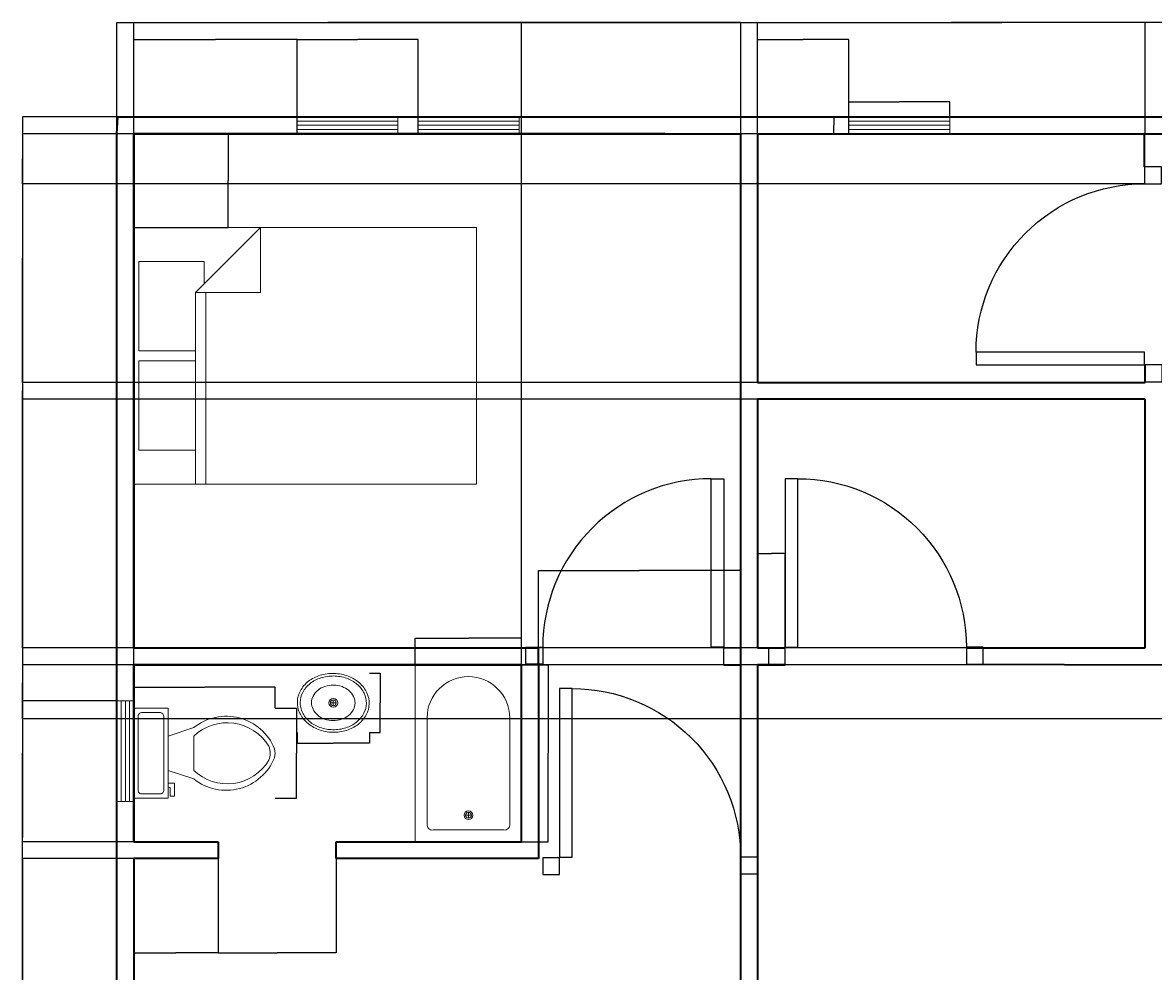
# Model space of a CAD drawing. Units: millimetres. Extents: x 1312 to 12932, y -881 to 10062.
# Tile 2 of 4: x 1312 to 8020, y 4434 to 10062. Entities that reach past the tile are written whole.
import ezdxf

# ---------------------------------------------------------------- set-up
doc = ezdxf.new("R2010")
doc.units = ezdxf.units.MM
for name, color, linetype, lineweight in [('A-ANNO-DIMS', 2, 'Continuous', 18), ('A-DOOR', 3, 'Continuous', 25), ('A-FLOR-FIXT', 9, 'Continuous', 18), ('A-FURN', 8, 'Continuous', 18), ('A-GLAZ', 4, 'Continuous', 18), ('A-WALL', 7, 'Continuous', 35)]:
    doc.layers.add(name, color=color, linetype=linetype, lineweight=lineweight)
doc.styles.get("Standard").update_dxf_attribs({"font": 'arial.ttf'})
doc.dimstyles.get("Standard").update_dxf_attribs({"dimtxt": 0.18, "dimasz": 0.18, "dimexe": 0.18, "dimexo": 0.0625, "dimgap": 0.09, "dimtad": 0, "dimtih": 1, "dimtoh": 1, "dimdec": 4, "dimzin": 0, "dimdsep": 46, "dimtxsty": 'Standard', "dimcen": 0.09, "dimadec": 0, "dimazin": 0, "dimtfac": 1, "dimtdec": 4, "dimtofl": 0, "dimtmove": 0, "dimatfit": 3, "dimfxl": 1, "dimtolj": 1, "dimtzin": 0, "dimarcsym": 0})

# ---------------------------------------------------------------- blocks, each defined once
blk = doc.blocks.new('Toilet - top')
for p, q in [((9.5, -6), (9.5, -2)), ((-10, -8.5), (-8, -8.5)), ((-10, -9.5), (-10, -8.5)), ((-7, -9.5), (-10, -9.5)), ((-8, -8.5), (-8, -8)), ((-7, -8), (-7, -9.5)), ((-4, -8), (-6, -14)), ((4, -8), (6, -14)), ((4, -14), (-4, -14))]:
    blk.add_line(p, q)
blk.add_lwpolyline([(10.5, -8), (10.5, 0), (-10.5, 0), (-10.5, -8)], close=True)
for points in [[(-9.5, -2), (-9.5, -6)], [(8.5, -1), (-8.5, -1)], [(-8.5, -7), (8.5, -7)]]:
    blk.add_lwpolyline(points)
for centre, radius, start, end in [((-8.62, -1.88), 0.884, 81.8699, 188.1301), ((8.62, -1.88), 0.884, 351.8699, 98.1301), ((-8.62, -6.12), 0.884, 171.8699, 278.1301), ((8.62, -6.12), 0.884, 261.8699, 8.1301), ((3.52, -21.58), 12.17, 141.4691, 247.9714), ((4.2, -21.82), 11.33, 136.3677, 238.9468), ((-3.52, -21.58), 12.17, 292.0284, 38.5307), ((-4.2, -21.82), 11.33, 301.053, 43.6321), ((0, -27.88), 4, 245.7318, 294.2682), ((0, -29), 4, 254.8605, 285.1395)]:
    blk.add_arc(centre, radius, start, end)
blk = doc.blocks.new('Bath Tub - 26 x 60 in.')
for p, q in [((8, -18), (10, -18)), ((9, -17), (9, -19))]:
    blk.add_line(p, q)
blk.add_lwpolyline([(0, -36), (0, 0), (60, 0), (60, -36)], close=True)
for points in [[(4, -30), (4, -6)], [(6, -4), (42, -4)], [(42, -32), (6, -32)]]:
    blk.add_lwpolyline(points)
for radius in [1.5, 1]:
    blk.add_circle((9, -18), radius)
for centre, radius, start, end in [((5.75, -5.75), 1.77, 81.8699, 188.1301), ((42, -18), 14, 270, 90), ((5.75, -30.25), 1.77, 171.8699, 278.1301)]:
    blk.add_arc(centre, radius, start, end)
blk = doc.blocks.new('Bed - Queen')
for p, q in [((0, -80.00003), (0, 0)), ((0, 0), (59.99999, 0)), ((59.99999, 0), (59.99999, -80.00003)), ((7.99999, -1.2), (28.79998, -1.2)), ((7.99999, -14.4), (7.99999, -1.2)), ((28.79998, -1.2), (28.79998, -14.4)), ((31.19999, -1.2), (51.99999, -1.2)), ((31.19999, -14.4), (31.19999, -1.2)), ((51.99999, -1.2), (51.99999, -16.4)), ((0, -14.4), (44.8, -14.4)), ((59.99999, -29.6), (44.8, -14.4)), ((44.8, -14.4), (44.8, -29.6)), ((44.8, -16.8), (0, -16.8)), ((51.99999, -16.4), (46.79936, -16.4)), ((44.8, -29.6), (59.99999, -29.6)), ((59.99999, -80.00003), (0, -80.00003))]:
    blk.add_line(p, q)
blk = doc.blocks.new('Sink - Oval top')
for p, q in [((-1, 0), (1, 0)), ((0, 1), (0, -1))]:
    blk.add_line(p, q)
for points in [[(-12.23, 0.39, 0.117634), (-11.46, -3.36, 0.104469), (-8.88, -6.8, 0.090016), (-5.08, -9.07, 0.08192), (-0.32, -10.02, 0.08192), (4.49, -9.38, 0.090016), (8.42, -7.36, 0.104469), (11.22, -4.09, 0.117634), (12.23, -0.39, 0.117634), (11.46, 3.36, 0.104469), (8.88, 6.8, 0.090016), (5.08, 9.07, 0.08192), (0.32, 10.02, 0.08192), (-4.49, 9.38, 0.090016), (-8.42, 7.36, 0.104469), (-11.22, 4.09, 0.117634)], [(-11.29, 0.16, 0.118622), (-10.52, -3.25, 0.104678), (-8.07, -6.36, 0.089562), (-4.54, -8.37, 0.081185), (-0.13, -9.15, 0.081185), (4.3, -8.49, 0.089562), (7.89, -6.58, 0.104678), (10.42, -3.55, 0.118622), (11.29, -0.16, 0.118622), (10.52, 3.25, 0.104678), (8.07, 6.36, 0.089562), (4.54, 8.37, 0.081185), (0.13, 9.15, 0.081185), (-4.3, 8.49, 0.089562), (-7.89, 6.58, 0.104678), (-10.42, 3.55, 0.118622)], [(-7.42, 0.08, 0.118283), (-6.91, -2.17, 0.104607), (-5.29, -4.21, 0.089718), (-2.97, -5.53, 0.081436), (-0.07, -6.04, 0.081436), (2.84, -5.59, 0.089718), (5.2, -4.33, 0.104607), (6.86, -2.32, 0.118283), (7.42, -0.08, 0.118283), (6.91, 2.17, 0.104607), (5.29, 4.21, 0.089718), (2.97, 5.53, 0.081436), (0.07, 6.04, 0.081436), (-2.84, 5.59, 0.089718), (-5.2, 4.33, 0.104607), (-6.86, 2.32, 0.118283)]]:
    blk.add_lwpolyline(points, format="xyb", close=True)
for radius in [1.5, 1]:
    blk.add_circle((0, 0), radius)
blk = doc.blocks.new('Window - Wood Frame 36 in. Wide plan')
for p, q in [((0, 6), (0, 0)), ((0, 4.5), (36, 4.5)), ((36, 6), (36, 0)), ((0, 3), (36, 3)), ((0, 1.5), (36, 1.5))]:
    blk.add_line(p, q)
blk = doc.blocks.new('DOOR-SINGLE-1000')
for p, q in [((0, 1003.8), (0, 1103.8)), ((0, 1103.8), (100, 1103.8)), ((100, 1103.8), (100, 1003.8)), ((1174.2, 1000), (1174.2, 1100)), ((1174.2, 1100), (1274.2, 1100)), ((1274.2, 1100), (1274.2, 1000)), ((100, 1003.8), (0, 1003.8)), ((100, 1000), (174.2, 1000)), ((100, 0), (100, 1000)), ((174.2, 1000), (174.2, 0)), ((1274.2, 1000), (1174.2, 1000)), ((174.2, 0), (100, 0))]:
    blk.add_line(p, q)
blk.add_arc((174.2, 1000), 1000, 270, 0)
blk = doc.blocks.new('*D13')
at = {"layer": 'A-ANNO-DIMS', "color": 0, "lineweight": -2, "transparency": 16777216}
for p, q in [((6214.3, 9503.1), (6214.3, 9593)), ((6214.4, 9592.8), (6512.1, 9592.8)), ((6812.1, 9592.8), (6514.5, 9592.8)), ((6812.3, 9503.1), (6812.3, 9593))]:
    blk.add_line(p, q, dxfattribs=at)
at = {"layer": 'A-ANNO-DIMS', "color": 0, "transparency": 16777216}
for points in [[(6214.4, 9592.8), (6214.4, 9592.7), (6214.3, 9592.8)], [(6812.1, 9592.8), (6812.1, 9592.7), (6812.3, 9592.8)]]:
    blk.add_solid(points, dxfattribs=at)
at = {"layer": 'Defpoints', "color": 0, "transparency": 16777216}
for p in [(6812.3, 9592.8), (6214.3, 9503.1), (6812.3, 9503.1)]:
    blk.add_point(p, dxfattribs=at)
at = {"layer": 'A-ANNO-DIMS', "color": 0, "transparency": 16777216, "insert": (6513.3, 9592.8), "char_height": 0.18, "attachment_point": 5}
blk.add_mtext('\\A1;WINDOW 598 TYP.', dxfattribs=at)
blk = doc.blocks.new('*D14')
at = {"layer": 'A-ANNO-DIMS', "color": 0, "lineweight": -2, "transparency": 16777216}
for p, q in [((6214.2, 9503.1), (6124.4, 9503.1)), ((6124.5, 9502.9), (6124.5, 9453.4)), ((6214.2, 9403.4), (6124.4, 9403.4)), ((6124.5, 9403.6), (6124.5, 9453))]:
    blk.add_line(p, q, dxfattribs=at)
at = {"layer": 'A-ANNO-DIMS', "color": 0, "transparency": 16777216}
for points in [[(6124.5, 9502.9), (6124.6, 9502.9), (6124.5, 9503.1)], [(6124.5, 9403.6), (6124.6, 9403.6), (6124.5, 9403.4)]]:
    blk.add_solid(points, dxfattribs=at)
at = {"layer": 'Defpoints', "color": 0, "transparency": 16777216}
for p in [(6124.5, 9503.1), (6214.3, 9503.1), (6214.3, 9403.4)]:
    blk.add_point(p, dxfattribs=at)
at = {"layer": 'A-ANNO-DIMS', "color": 0, "transparency": 16777216, "insert": (6124.5, 9453.2), "char_height": 0.18, "attachment_point": 5}
blk.add_mtext('\\A1;100 TYP.', dxfattribs=at)
blk = doc.blocks.new('*D21')
at = {"layer": 'A-ANNO-DIMS', "color": 0, "lineweight": -2, "transparency": 16777216}
for p, q in [((1972, 5994.8), (1972, 6120.8)), ((1972.2, 6120.7), (2390.8, 6120.7)), ((2811.2, 6120.7), (2392.5, 6120.7)), ((2811.4, 5994.8), (2811.4, 6120.8))]:
    blk.add_line(p, q, dxfattribs=at)
at = {"layer": 'A-ANNO-DIMS', "color": 0, "transparency": 16777216}
for points in [[(1972.2, 6120.7), (1972.2, 6120.6), (1972, 6120.7)], [(2811.2, 6120.7), (2811.2, 6120.6), (2811.4, 6120.7)]]:
    blk.add_solid(points, dxfattribs=at)
at = {"layer": 'Defpoints', "color": 0, "transparency": 16777216}
for p in [(1972, 6120.7), (1972, 5994.8), (2811.4, 5994.8)]:
    blk.add_point(p, dxfattribs=at)
at = {"layer": 'A-ANNO-DIMS', "color": 0, "transparency": 16777216, "insert": (2391.7, 6120.7), "char_height": 0.18, "attachment_point": 5}
blk.add_mtext('\\A1;WC 839 TYP.', dxfattribs=at)
blk = doc.blocks.new('*D22')
at = {"layer": 'A-ANNO-DIMS', "color": 0, "lineweight": -2, "transparency": 16777216}
for p, q in [((2811.4, 5994.8), (2937.5, 5994.8)), ((2937.3, 5994.6), (2937.3, 5728.2)), ((2937.3, 5461.5), (2937.3, 5727.9)), ((2811.4, 5461.4), (2937.5, 5461.4))]:
    blk.add_line(p, q, dxfattribs=at)
at = {"layer": 'A-ANNO-DIMS', "color": 0, "transparency": 16777216}
for points in [[(2937.2, 5994.6), (2937.3, 5994.6), (2937.3, 5994.8)], [(2937.2, 5461.5), (2937.3, 5461.5), (2937.3, 5461.4)]]:
    blk.add_solid(points, dxfattribs=at)
at = {"layer": 'Defpoints', "color": 0, "transparency": 16777216}
for p in [(2811.4, 5994.8), (2937.3, 5994.8), (2811.4, 5461.4)]:
    blk.add_point(p, dxfattribs=at)
at = {"layer": 'A-ANNO-DIMS', "color": 0, "transparency": 16777216, "insert": (2937.3, 5728.1), "char_height": 0.18, "attachment_point": 5}
blk.add_mtext('\\A1;533 TYP.', dxfattribs=at)
blk = doc.blocks.new('*D23')
at = {"layer": 'A-ANNO-DIMS', "color": 0, "lineweight": -2, "transparency": 16777216}
for p, q in [((4272.1, 6253.1), (4429.7, 6253.1)), ((4429.5, 6252.9), (4429.5, 5728.2)), ((4429.5, 5203.2), (4429.5, 5727.9)), ((4272.1, 5203.1), (4429.7, 5203.1))]:
    blk.add_line(p, q, dxfattribs=at)
at = {"layer": 'A-ANNO-DIMS', "color": 0, "transparency": 16777216}
for points in [[(4429.5, 6252.9), (4429.5, 6252.9), (4429.5, 6253.1)], [(4429.5, 5203.2), (4429.5, 5203.2), (4429.5, 5203.1)]]:
    blk.add_solid(points, dxfattribs=at)
at = {"layer": 'Defpoints', "color": 0, "transparency": 16777216}
for p in [(4272, 6253.1), (4429.5, 6253.1), (4272, 5203.1)]:
    blk.add_point(p, dxfattribs=at)
at = {"layer": 'A-ANNO-DIMS', "color": 0, "transparency": 16777216, "insert": (4429.5, 5728.1), "char_height": 0.18, "attachment_point": 5}
blk.add_mtext('\\A1;BATH 1050', dxfattribs=at)
blk = doc.blocks.new('*D24')
at = {"layer": 'A-ANNO-DIMS', "color": 0, "lineweight": -2, "transparency": 16777216}
for p, q in [((3642, 6253.1), (3642, 6410.7)), ((3642.2, 6410.6), (3956.7, 6410.6)), ((4271.8, 6410.6), (3957.3, 6410.6)), ((4272, 6253.1), (4272, 6410.7))]:
    blk.add_line(p, q, dxfattribs=at)
at = {"layer": 'A-ANNO-DIMS', "color": 0, "transparency": 16777216}
for points in [[(3642.2, 6410.6), (3642.2, 6410.5), (3642, 6410.6)], [(4271.8, 6410.6), (4271.8, 6410.5), (4272, 6410.6)]]:
    blk.add_solid(points, dxfattribs=at)
at = {"layer": 'Defpoints', "color": 0, "transparency": 16777216}
for p in [(3642, 6410.6), (3642, 6253.1), (4272, 6253.1)]:
    blk.add_point(p, dxfattribs=at)
at = {"layer": 'A-ANNO-DIMS', "color": 0, "transparency": 16777216, "insert": (3957, 6410.6), "char_height": 0.18, "attachment_point": 5}
blk.add_mtext('\\A1;630', dxfattribs=at)
blk = doc.blocks.new('*D29')
at = {"layer": 'A-ANNO-DIMS', "color": 0, "lineweight": -2, "transparency": 16777216}
for p, q in [((2941.6, 5851.8), (2941.6, 5787.5)), ((3369.2, 5851.8), (3369.2, 5787.5)), ((2941.8, 5787.7), (3154.7, 5787.7)), ((3369, 5787.7), (3156.1, 5787.7))]:
    blk.add_line(p, q, dxfattribs=at)
at = {"layer": 'A-ANNO-DIMS', "color": 0, "transparency": 16777216}
for points in [[(2941.8, 5787.7), (2941.8, 5787.7), (2941.6, 5787.7)], [(3369, 5787.7), (3369, 5787.7), (3369.2, 5787.7)]]:
    blk.add_solid(points, dxfattribs=at)
at = {"layer": 'Defpoints', "color": 0, "transparency": 16777216}
for p in [(2941.6, 5851.8), (3369.2, 5851.8), (3369.2, 5787.7)]:
    blk.add_point(p, dxfattribs=at)
at = {"layer": 'A-ANNO-DIMS', "color": 0, "transparency": 16777216, "insert": (3155.4, 5787.7), "char_height": 0.18, "attachment_point": 5}
blk.add_mtext('\\A1;BASIN 428', dxfattribs=at)
blk = doc.blocks.new('*D30')
at = {"layer": 'A-ANNO-DIMS', "color": 0, "lineweight": -2, "transparency": 16777216}
for p, q in [((3369.2, 6202.5), (3433.5, 6202.5)), ((3433.3, 6202.4), (3433.3, 6027.4)), ((3433.3, 5852), (3433.3, 6027)), ((3369.2, 5851.8), (3433.5, 5851.8))]:
    blk.add_line(p, q, dxfattribs=at)
at = {"layer": 'A-ANNO-DIMS', "color": 0, "transparency": 16777216}
for points in [[(3433.3, 6202.4), (3433.3, 6202.4), (3433.3, 6202.5)], [(3433.3, 5852), (3433.3, 5852), (3433.3, 5851.8)]]:
    blk.add_solid(points, dxfattribs=at)
at = {"layer": 'Defpoints', "color": 0, "transparency": 16777216}
for p in [(3369.2, 6202.5), (3433.3, 6202.5), (3369.2, 5851.8)]:
    blk.add_point(p, dxfattribs=at)
at = {"layer": 'A-ANNO-DIMS', "color": 0, "transparency": 16777216, "insert": (3433.3, 6027.2), "char_height": 0.18, "attachment_point": 5}
blk.add_mtext('\\A1;351', dxfattribs=at)
blk = doc.blocks.new('*D41')
at = {"layer": 'A-ANNO-DIMS', "color": 0, "lineweight": -2, "transparency": 16777216}
for p, q in [((1872, 9403.1), (1872, 10062.5)), ((1872.2, 10062.3), (7121.6, 10062.3)), ((12371.8, 10062.3), (7122.4, 10062.3)), ((12372, 9503.1), (12372, 10062.5))]:
    blk.add_line(p, q, dxfattribs=at)
at = {"layer": 'A-ANNO-DIMS', "color": 0, "transparency": 16777216}
for points in [[(1872.2, 10062.3), (1872.2, 10062.3), (1872, 10062.3)], [(12371.8, 10062.3), (12371.8, 10062.3), (12372, 10062.3)]]:
    blk.add_solid(points, dxfattribs=at)
at = {"layer": 'Defpoints', "color": 0, "transparency": 16777216}
for p in [(12372, 10062.3), (12372, 9503.1), (1872, 9403.1)]:
    blk.add_point(p, dxfattribs=at)
at = {"layer": 'A-ANNO-DIMS', "color": 0, "transparency": 16777216, "insert": (7122, 10062.3), "char_height": 0.18, "attachment_point": 5}
blk.add_mtext('\\A1;10500', dxfattribs=at)
blk = doc.blocks.new('*D42')
at = {"layer": 'A-ANNO-DIMS', "color": 0, "lineweight": -2, "transparency": 16777216}
for p, q in [((1876.6, 9503.1), (1312.6, 9503.1)), ((1312.7, 9502.9), (1312.7, 5228.2)), ((1312.7, 953.2), (1312.7, 5227.9)), ((1871.9, 953.1), (1312.6, 953.1))]:
    blk.add_line(p, q, dxfattribs=at)
at = {"layer": 'A-ANNO-DIMS', "color": 0, "transparency": 16777216}
for points in [[(1312.7, 9502.9), (1312.8, 9502.9), (1312.7, 9503.1)], [(1312.7, 953.2), (1312.8, 953.2), (1312.7, 953.1)]]:
    blk.add_solid(points, dxfattribs=at)
at = {"layer": 'Defpoints', "color": 0, "transparency": 16777216}
for p in [(1312.7, 9503.1), (1876.6, 9503.1), (1872, 953.1)]:
    blk.add_point(p, dxfattribs=at)
at = {"layer": 'A-ANNO-DIMS', "color": 0, "transparency": 16777216, "insert": (1312.7, 5228.1), "char_height": 0.18, "attachment_point": 5}
blk.add_mtext('\\A1;8550', dxfattribs=at)
blk = doc.blocks.new('*D43')
at = {"layer": 'A-ANNO-DIMS', "color": 0, "lineweight": -2, "transparency": 16777216}
for p, q in [((1972, 9403.1), (1972, 10062.5)), ((1972.2, 10062.3), (3771.6, 10062.3)), ((5571.8, 10062.3), (3772.4, 10062.3)), ((5572, 9403.1), (5572, 10062.5))]:
    blk.add_line(p, q, dxfattribs=at)
at = {"layer": 'A-ANNO-DIMS', "color": 0, "transparency": 16777216}
for points in [[(1972.2, 10062.3), (1972.2, 10062.3), (1972, 10062.3)], [(5571.8, 10062.3), (5571.8, 10062.3), (5572, 10062.3)]]:
    blk.add_solid(points, dxfattribs=at)
at = {"layer": 'Defpoints', "color": 0, "transparency": 16777216}
for p in [(5572, 10062.3), (1972, 9403.1), (5572, 9403.1)]:
    blk.add_point(p, dxfattribs=at)
at = {"layer": 'A-ANNO-DIMS', "color": 0, "transparency": 16777216, "insert": (3772, 10062.3), "char_height": 0.18, "attachment_point": 5}
blk.add_mtext('\\A1;3600', dxfattribs=at)
blk = doc.blocks.new('*D44')
at = {"layer": 'A-ANNO-DIMS', "color": 0, "lineweight": -2, "transparency": 16777216}
for p, q in [((5671.992231, 9403.123661), (5671.992231, 10062.491161)), ((5672.172231, 10062.311161), (6821.632231, 10062.311161)), ((7971.812231, 10062.311161), (6822.352231, 10062.311161)), ((7971.992231, 9403.123661), (7971.992231, 10062.491161))]:
    blk.add_line(p, q, dxfattribs=at)
at = {"layer": 'A-ANNO-DIMS', "color": 0, "transparency": 16777216}
for points in [[(5672.172231, 10062.341161), (5672.172231, 10062.281161), (5671.992231, 10062.311161)], [(7971.812231, 10062.341161), (7971.812231, 10062.281161), (7971.992231, 10062.311161)]]:
    blk.add_solid(points, dxfattribs=at)
at = {"layer": 'Defpoints', "color": 0, "transparency": 16777216}
for p in [(7971.992231, 10062.311161), (5671.992231, 9403.061161), (7971.992231, 9403.061161)]:
    blk.add_point(p, dxfattribs=at)
at = {"layer": 'A-ANNO-DIMS', "color": 0, "transparency": 16777216, "insert": (6821.992231, 10062.311161), "char_height": 0.18, "attachment_point": 5}
blk.add_mtext('\\A1;2300', dxfattribs=at)
blk = doc.blocks.new('*D47')
at = {"layer": 'A-ANNO-DIMS', "color": 0, "lineweight": -2, "transparency": 16777216}
for p, q in [((1971.9, 5103.1), (1312.6, 5103.1)), ((1312.7, 5102.9), (1312.7, 3078.2)), ((1312.7, 1053.2), (1312.7, 3077.9)), ((1971.9, 1053.1), (1312.6, 1053.1))]:
    blk.add_line(p, q, dxfattribs=at)
at = {"layer": 'A-ANNO-DIMS', "color": 0, "transparency": 16777216}
for points in [[(1312.7, 5102.9), (1312.8, 5102.9), (1312.7, 5103.1)], [(1312.7, 1053.2), (1312.8, 1053.2), (1312.7, 1053.1)]]:
    blk.add_solid(points, dxfattribs=at)
at = {"layer": 'Defpoints', "color": 0, "transparency": 16777216}
for p in [(1312.7, 5103.1), (1972, 5103.1), (1972, 1053.1)]:
    blk.add_point(p, dxfattribs=at)
at = {"layer": 'A-ANNO-DIMS', "color": 0, "transparency": 16777216, "insert": (1312.7, 3078.1), "char_height": 0.18, "attachment_point": 5}
blk.add_mtext('\\A1;4050', dxfattribs=at)
blk = doc.blocks.new('*D48')
at = {"layer": 'A-ANNO-DIMS', "color": 0, "lineweight": -2, "transparency": 16777216}
for p, q in [((1971.9, 6253.1), (1312.6, 6253.1)), ((1312.7, 6252.9), (1312.7, 5728.2)), ((1312.7, 5203.2), (1312.7, 5727.9)), ((1971.9, 5203.1), (1312.6, 5203.1))]:
    blk.add_line(p, q, dxfattribs=at)
at = {"layer": 'A-ANNO-DIMS', "color": 0, "transparency": 16777216}
for points in [[(1312.7, 6252.9), (1312.8, 6252.9), (1312.7, 6253.1)], [(1312.7, 5203.2), (1312.8, 5203.2), (1312.7, 5203.1)]]:
    blk.add_solid(points, dxfattribs=at)
at = {"layer": 'Defpoints', "color": 0, "transparency": 16777216}
for p in [(1312.7, 6253.1), (1972, 6253.1), (1972, 5203.1)]:
    blk.add_point(p, dxfattribs=at)
at = {"layer": 'A-ANNO-DIMS', "color": 0, "transparency": 16777216, "insert": (1312.7, 5728.1), "char_height": 0.18, "attachment_point": 5}
blk.add_mtext('\\A1;1050', dxfattribs=at)
blk = doc.blocks.new('*D49')
at = {"layer": 'A-ANNO-DIMS', "color": 0, "lineweight": -2, "transparency": 16777216}
for p, q in [((1971.9, 9403.1), (1312.6, 9403.1)), ((1312.7, 9402.9), (1312.7, 7878.2)), ((1312.7, 6353.2), (1312.7, 7877.9)), ((1971.9, 6353.1), (1312.6, 6353.1))]:
    blk.add_line(p, q, dxfattribs=at)
at = {"layer": 'A-ANNO-DIMS', "color": 0, "transparency": 16777216}
for points in [[(1312.7, 9402.9), (1312.8, 9402.9), (1312.7, 9403.1)], [(1312.7, 6353.2), (1312.8, 6353.2), (1312.7, 6353.1)]]:
    blk.add_solid(points, dxfattribs=at)
at = {"layer": 'Defpoints', "color": 0, "transparency": 16777216}
for p in [(1312.7, 9403.1), (1972, 9403.1), (1972, 6353.1)]:
    blk.add_point(p, dxfattribs=at)
at = {"layer": 'A-ANNO-DIMS', "color": 0, "transparency": 16777216, "insert": (1312.7, 7878.1), "char_height": 0.18, "attachment_point": 5}
blk.add_mtext('\\A1;3050', dxfattribs=at)
blk = doc.blocks.new('*D50')
at = {"layer": 'A-ANNO-DIMS', "color": 0, "lineweight": -2, "transparency": 16777216}
for p, q in [((4372, 6253.1), (4372, 6812.5)), ((4372.2, 6812.3), (4971.6, 6812.3)), ((5571.8, 6812.3), (4972.3, 6812.3)), ((5572, 6253.1), (5572, 6812.5))]:
    blk.add_line(p, q, dxfattribs=at)
at = {"layer": 'A-ANNO-DIMS', "color": 0, "transparency": 16777216}
for points in [[(4372.2, 6812.3), (4372.2, 6812.3), (4372, 6812.3)], [(5571.8, 6812.3), (5571.8, 6812.3), (5572, 6812.3)]]:
    blk.add_solid(points, dxfattribs=at)
at = {"layer": 'Defpoints', "color": 0, "transparency": 16777216}
for p in [(5572, 6812.3), (4372, 6253.1), (5572, 6253.1)]:
    blk.add_point(p, dxfattribs=at)
at = {"layer": 'A-ANNO-DIMS', "color": 0, "transparency": 16777216, "insert": (4972, 6812.3), "char_height": 0.18, "attachment_point": 5}
blk.add_mtext('\\A1;1200', dxfattribs=at)
blk = doc.blocks.new('*D54')
at = {"layer": 'A-ANNO-DIMS', "color": 0, "lineweight": -2, "transparency": 16777216}
for p, q in [((7971.9, 9403.1), (1312.6, 9403.1)), ((1312.7, 9402.9), (1312.7, 8665.7)), ((1312.7, 7928.2), (1312.7, 8665.4)), ((7971.9, 7928.1), (1312.6, 7928.1))]:
    blk.add_line(p, q, dxfattribs=at)
at = {"layer": 'A-ANNO-DIMS', "color": 0, "transparency": 16777216}
for points in [[(1312.7, 9402.9), (1312.8, 9402.9), (1312.7, 9403.1)], [(1312.7, 7928.2), (1312.8, 7928.2), (1312.7, 7928.1)]]:
    blk.add_solid(points, dxfattribs=at)
at = {"layer": 'Defpoints', "color": 0, "transparency": 16777216}
for p in [(7972, 9403.1), (1312.7, 7928.1), (7972, 7928.1)]:
    blk.add_point(p, dxfattribs=at)
at = {"layer": 'A-ANNO-DIMS', "color": 0, "transparency": 16777216, "insert": (1312.7, 8665.6), "char_height": 0.18, "attachment_point": 5}
blk.add_mtext('\\A1;1475', dxfattribs=at)
blk = doc.blocks.new('*D55')
at = {"layer": 'A-ANNO-DIMS', "color": 0, "lineweight": -2, "transparency": 16777216}
for p, q in [((7971.9, 7828.1), (1312.6, 7828.1)), ((1312.7, 7827.9), (1312.7, 7090.7)), ((1312.7, 6353.2), (1312.7, 7090.4)), ((7971.9, 6353.1), (1312.6, 6353.1))]:
    blk.add_line(p, q, dxfattribs=at)
at = {"layer": 'A-ANNO-DIMS', "color": 0, "transparency": 16777216}
for points in [[(1312.7, 7827.9), (1312.8, 7827.9), (1312.7, 7828.1)], [(1312.7, 6353.2), (1312.8, 6353.2), (1312.7, 6353.1)]]:
    blk.add_solid(points, dxfattribs=at)
at = {"layer": 'Defpoints', "color": 0, "transparency": 16777216}
for p in [(7972, 7828.1), (1312.7, 6353.1), (7972, 6353.1)]:
    blk.add_point(p, dxfattribs=at)
at = {"layer": 'A-ANNO-DIMS', "color": 0, "transparency": 16777216, "insert": (1312.7, 7090.6), "char_height": 0.18, "attachment_point": 5}
blk.add_mtext('\\A1;1475', dxfattribs=at)
blk = doc.blocks.new('*D64')
at = {"layer": 'A-ANNO-DIMS', "color": 0, "lineweight": -2, "transparency": 16777216}
for p, q in [((1972, 9403.1), (1971.8, 9962.5)), ((1972, 9962.3), (2456, 9962.5)), ((2940.6, 9962.6), (2456.6, 9962.5)), ((2940.9, 9403.4), (2940.7, 9962.8))]:
    blk.add_line(p, q, dxfattribs=at)
at = {"layer": 'A-ANNO-DIMS', "color": 0, "transparency": 16777216}
for points in [[(1972, 9962.3), (1972, 9962.3), (1971.8, 9962.3)], [(2940.6, 9962.7), (2940.6, 9962.6), (2940.7, 9962.6)]]:
    blk.add_solid(points, dxfattribs=at)
at = {"layer": 'Defpoints', "color": 0, "transparency": 16777216}
for p in [(2940.7, 9962.6), (1972, 9403.1), (2940.9, 9403.4)]:
    blk.add_point(p, dxfattribs=at)
at = {"layer": 'A-ANNO-DIMS', "color": 0, "transparency": 16777216, "insert": (2456.3, 9962.5), "char_height": 0.18, "attachment_point": 5}
blk.add_mtext('\\A1;969', dxfattribs=at)
blk = doc.blocks.new('*D65')
at = {"layer": 'A-ANNO-DIMS', "color": 0, "lineweight": -2, "transparency": 16777216}
for p, q in [((2940.9, 9403.4), (2940.9, 9962.8)), ((2941.1, 9962.6), (3299.7, 9962.6)), ((3658.8, 9962.6), (3300.2, 9962.6)), ((3659, 9403.4), (3659, 9962.8))]:
    blk.add_line(p, q, dxfattribs=at)
at = {"layer": 'A-ANNO-DIMS', "color": 0, "transparency": 16777216}
for points in [[(2941.1, 9962.7), (2941.1, 9962.6), (2940.9, 9962.6)], [(3658.8, 9962.7), (3658.8, 9962.6), (3659, 9962.6)]]:
    blk.add_solid(points, dxfattribs=at)
at = {"layer": 'Defpoints', "color": 0, "transparency": 16777216}
for p in [(3659, 9962.6), (2940.9, 9403.4), (3659, 9403.4)]:
    blk.add_point(p, dxfattribs=at)
at = {"layer": 'A-ANNO-DIMS', "color": 0, "transparency": 16777216, "insert": (3300, 9962.6), "char_height": 0.18, "attachment_point": 5}
blk.add_mtext('\\A1;718', dxfattribs=at)
blk = doc.blocks.new('*D66')
at = {"layer": 'A-ANNO-DIMS', "color": 0, "lineweight": -2, "transparency": 16777216}
for p, q in [((5672, 9403.1), (5671.7, 9962.5)), ((5671.8, 9962.3), (5942.4, 9962.5)), ((6213.7, 9962.6), (5943.2, 9962.5)), ((6214.3, 9403.4), (6213.9, 9962.8))]:
    blk.add_line(p, q, dxfattribs=at)
at = {"layer": 'A-ANNO-DIMS', "color": 0, "transparency": 16777216}
for points in [[(5671.8, 9962.3), (5671.8, 9962.3), (5671.7, 9962.3)], [(6213.7, 9962.7), (6213.7, 9962.6), (6213.9, 9962.6)]]:
    blk.add_solid(points, dxfattribs=at)
at = {"layer": 'Defpoints', "color": 0, "transparency": 16777216}
for p in [(6213.9, 9962.6), (5672, 9403.1), (6214.3, 9403.4)]:
    blk.add_point(p, dxfattribs=at)
at = {"layer": 'A-ANNO-DIMS', "color": 0, "transparency": 16777216, "insert": (5942.8, 9962.5), "char_height": 0.18, "attachment_point": 5}
blk.add_mtext('\\A1;542.3', dxfattribs=at)
blk = doc.blocks.new('*D77')
at = {"layer": 'A-ANNO-DIMS', "color": 0, "lineweight": -2, "transparency": 16777216}
for p, q in [((1971.9, 6253.1), (1312.6, 6253.1)), ((1312.7, 6252.9), (1312.7, 6146.6)), ((1312.7, 6039.9), (1312.7, 6146.2)), ((1872.3, 6039.8), (1312.6, 6039.8))]:
    blk.add_line(p, q, dxfattribs=at)
at = {"layer": 'A-ANNO-DIMS', "color": 0, "transparency": 16777216}
for points in [[(1312.7, 6252.9), (1312.8, 6252.9), (1312.7, 6253.1)], [(1312.7, 6039.9), (1312.8, 6039.9), (1312.7, 6039.8)]]:
    blk.add_solid(points, dxfattribs=at)
at = {"layer": 'Defpoints', "color": 0, "transparency": 16777216}
for p in [(1312.7, 6253.1), (1972, 6253.1), (1872.3, 6039.8)]:
    blk.add_point(p, dxfattribs=at)
at = {"layer": 'A-ANNO-DIMS', "color": 0, "transparency": 16777216, "insert": (1312.7, 6146.4), "char_height": 0.18, "attachment_point": 5}
blk.add_mtext('\\A1;213.3', dxfattribs=at)
blk = doc.blocks.new('*D78')
at = {"layer": 'A-ANNO-DIMS', "color": 0, "lineweight": -2, "transparency": 16777216}
for p, q in [((2472, 5103), (2472, 4543.6)), ((3172, 5103), (3172, 4543.6)), ((2472.2, 4543.8), (2821.7, 4543.8)), ((3171.8, 4543.8), (2822.3, 4543.8))]:
    blk.add_line(p, q, dxfattribs=at)
at = {"layer": 'A-ANNO-DIMS', "color": 0, "transparency": 16777216}
for points in [[(2472.2, 4543.8), (2472.2, 4543.8), (2472, 4543.8)], [(3171.8, 4543.8), (3171.8, 4543.8), (3172, 4543.8)]]:
    blk.add_solid(points, dxfattribs=at)
at = {"layer": 'Defpoints', "color": 0, "transparency": 16777216}
for p in [(2472, 5103.1), (3172, 5103.1), (2472, 4543.8)]:
    blk.add_point(p, dxfattribs=at)
at = {"layer": 'A-ANNO-DIMS', "color": 0, "transparency": 16777216, "insert": (2822, 4543.8), "char_height": 0.18, "attachment_point": 5}
blk.add_mtext('\\A1;700', dxfattribs=at)
blk = doc.blocks.new('*D79')
at = {"layer": 'A-ANNO-DIMS', "color": 0, "lineweight": -2, "transparency": 16777216}
for p, q in [((1972, 5103), (1972, 4543.6)), ((2472, 5103), (2472, 4543.6)), ((1972.2, 4543.8), (2221.7, 4543.8)), ((2471.8, 4543.8), (2222.3, 4543.8))]:
    blk.add_line(p, q, dxfattribs=at)
at = {"layer": 'A-ANNO-DIMS', "color": 0, "transparency": 16777216}
for points in [[(1972.2, 4543.8), (1972.2, 4543.8), (1972, 4543.8)], [(2471.8, 4543.8), (2471.8, 4543.8), (2472, 4543.8)]]:
    blk.add_solid(points, dxfattribs=at)
at = {"layer": 'Defpoints', "color": 0, "transparency": 16777216}
for p in [(1972, 5103.1), (2472, 5103.1), (1972, 4543.8)]:
    blk.add_point(p, dxfattribs=at)
at = {"layer": 'A-ANNO-DIMS', "color": 0, "transparency": 16777216, "insert": (2222, 4543.8), "char_height": 0.18, "attachment_point": 5}
blk.add_mtext('\\A1;500', dxfattribs=at)
blk = doc.blocks.new('*D82')
at = {"layer": 'A-ANNO-DIMS', "color": 0, "lineweight": -2, "transparency": 16777216}
for p, q in [((1972.1, 9403.1), (2531.4, 9403.1)), ((2531.2, 9402.9), (2531.2, 9125.6)), ((2531.2, 8848), (2531.2, 9125.3)), ((1972.1, 8847.8), (2531.4, 8847.8))]:
    blk.add_line(p, q, dxfattribs=at)
at = {"layer": 'A-ANNO-DIMS', "color": 0, "transparency": 16777216}
for points in [[(2531.2, 9402.9), (2531.3, 9402.9), (2531.2, 9403.1)], [(2531.2, 8848), (2531.3, 8848), (2531.2, 8847.8)]]:
    blk.add_solid(points, dxfattribs=at)
at = {"layer": 'Defpoints', "color": 0, "transparency": 16777216}
for p in [(1972, 9403.1), (1972, 8847.8), (2531.2, 8847.8)]:
    blk.add_point(p, dxfattribs=at)
at = {"layer": 'A-ANNO-DIMS', "color": 0, "transparency": 16777216, "insert": (2531.2, 9125.5), "char_height": 0.18, "attachment_point": 5}
blk.add_mtext('\\A1;555.2', dxfattribs=at)
blk = doc.blocks.new('*D84')
at = {"layer": 'A-ANNO-DIMS', "color": 0, "lineweight": -2, "transparency": 16777216}
for p, q in [((5672, 6353.1), (5672, 6912.5)), ((5672.2, 6912.3), (5753.9, 6912.3)), ((5836.6, 6912.3), (5754.8, 6912.3)), ((5836.8, 6353.1), (5836.8, 6912.5))]:
    blk.add_line(p, q, dxfattribs=at)
at = {"layer": 'A-ANNO-DIMS', "color": 0, "transparency": 16777216}
for points in [[(5672.2, 6912.3), (5672.2, 6912.3), (5672, 6912.3)], [(5836.6, 6912.3), (5836.6, 6912.3), (5836.8, 6912.3)]]:
    blk.add_solid(points, dxfattribs=at)
at = {"layer": 'Defpoints', "color": 0, "transparency": 16777216}
for p in [(5836.8, 6912.3), (5672, 6353.1), (5836.8, 6353.1)]:
    blk.add_point(p, dxfattribs=at)
at = {"layer": 'A-ANNO-DIMS', "color": 0, "transparency": 16777216, "insert": (5754.4, 6912.3), "char_height": 0.18, "attachment_point": 5}
blk.add_mtext('\\A1;164.76', dxfattribs=at)
blk = doc.blocks.new('*D85')
at = {"layer": 'A-ANNO-DIMS', "color": 0, "lineweight": -2, "transparency": 16777216}
for p, q in [((1971.992231, 5203.123661), (1971.992231, 10062.491161)), ((1972.172231, 10062.311161), (3121.632231, 10062.311161)), ((4271.812231, 10062.311161), (3122.352231, 10062.311161)), ((4271.992231, 5203.123661), (4271.992231, 10062.491161))]:
    blk.add_line(p, q, dxfattribs=at)
at = {"layer": 'A-ANNO-DIMS', "color": 0, "transparency": 16777216}
for points in [[(1972.172231, 10062.341161), (1972.172231, 10062.281161), (1971.992231, 10062.311161)], [(4271.812231, 10062.341161), (4271.812231, 10062.281161), (4271.992231, 10062.311161)]]:
    blk.add_solid(points, dxfattribs=at)
at = {"layer": 'Defpoints', "color": 0, "transparency": 16777216}
for p in [(4271.992231, 10062.311161), (1971.992231, 5203.061161), (4271.992231, 5203.061161)]:
    blk.add_point(p, dxfattribs=at)
at = {"layer": 'A-ANNO-DIMS', "color": 0, "transparency": 16777216, "insert": (3121.992231, 10062.311161), "char_height": 0.18, "attachment_point": 5}
blk.add_mtext('\\A1;2300', dxfattribs=at)
blk = doc.blocks.new('*D86')
at = {"layer": 'A-ANNO-DIMS', "color": 0, "lineweight": -2, "transparency": 16777216}
for p, q in [((7971.9, 9403.1), (1312.6, 9403.1)), ((1312.7, 9402.9), (1312.7, 9255)), ((1312.7, 9106.8), (1312.7, 9254.7)), ((7968.2, 9106.7), (1312.6, 9106.7))]:
    blk.add_line(p, q, dxfattribs=at)
at = {"layer": 'A-ANNO-DIMS', "color": 0, "transparency": 16777216}
for points in [[(1312.7, 9402.9), (1312.8, 9402.9), (1312.7, 9403.1)], [(1312.7, 9106.8), (1312.8, 9106.8), (1312.7, 9106.7)]]:
    blk.add_solid(points, dxfattribs=at)
at = {"layer": 'Defpoints', "color": 0, "transparency": 16777216}
for p in [(7972, 9403.1), (1312.7, 9106.7), (7968.2, 9106.7)]:
    blk.add_point(p, dxfattribs=at)
at = {"layer": 'A-ANNO-DIMS', "color": 0, "transparency": 16777216, "insert": (1312.7, 9254.9), "char_height": 0.18, "attachment_point": 5}
blk.add_mtext('\\A1;296.4', dxfattribs=at)
blk = doc.blocks.new('*D94')
at = {"layer": 'A-ANNO-DIMS', "color": 0, "lineweight": -2, "transparency": 16777216}
for p, q in [((9571.9, 6253.1), (1312.6, 6253.1)), ((1312.7, 6252.9), (1312.7, 6093.4)), ((1312.7, 5933.5), (1312.7, 6093)), ((9848.9, 5933.3), (1312.6, 5933.3))]:
    blk.add_line(p, q, dxfattribs=at)
at = {"layer": 'A-ANNO-DIMS', "color": 0, "transparency": 16777216}
for points in [[(1312.7, 6252.9), (1312.8, 6252.9), (1312.7, 6253.1)], [(1312.7, 5933.5), (1312.8, 5933.5), (1312.7, 5933.3)]]:
    blk.add_solid(points, dxfattribs=at)
at = {"layer": 'Defpoints', "color": 0, "transparency": 16777216}
for p in [(1312.7, 6253.1), (9572, 6253.1), (9849, 5933.3)]:
    blk.add_point(p, dxfattribs=at)
at = {"layer": 'A-ANNO-DIMS', "color": 0, "transparency": 16777216, "insert": (1312.7, 6093.2), "char_height": 0.18, "attachment_point": 5}
blk.add_mtext('\\A1;319.7', dxfattribs=at)

msp = doc.modelspace()

# ---------------------------------------------------------------- linework, layer by layer
at = {"layer": 'A-DOOR'}
msp.add_line((5910.956, 7356.829), (5836.756, 7356.829), dxfattribs=at)
at = {"layer": 'A-WALL'}
for p, q in [((1871.992, 9403.061), (1876.635, 9503.061)), ((1876.635, 9503.061), (12371.992, 9503.061)), ((1971.992, 9503.061), (5121.992, 9503.061)), ((1871.992, 953.061), (1871.992, 9403.061)), ((1971.992, 6353.061), (1971.992, 9403.061)), ((1971.992, 9403.061), (5571.992, 9403.061)), ((1971.992, 9403.061), (1971.992, 6353.061)), ((5121.992, 9403.061), (1971.992, 9403.061)), ((5571.992, 1053.061), (5571.992, 9403.061)), ((5671.992, 9403.061), (5671.992, 7928.061)), ((5671.992, 9403.061), (6871.992, 9403.061)), ((6871.992, 9403.061), (7971.992, 9403.061)), ((7968.224, 9206.669), (7968.224, 9403.061)), ((7968.224, 9403.061), (8071.992, 9403.061)), ((5671.992, 8603.061), (5671.992, 7928.061)), ((7971.992, 7928.061), (7971.992, 8032.469)), ((5671.992, 7928.061), (7971.992, 7928.061)), ((7971.992, 7828.061), (5671.992, 7828.061)), ((7971.992, 7828.061), (5671.992, 7828.061)), ((5671.992, 7828.061), (5671.992, 7628.061)), ((5671.992, 7828.061), (5671.992, 6353.061)), ((7971.992, 6353.061), (7971.992, 7828.061)), ((1971.992, 6353.061), (4371.992, 6353.061)), ((4371.992, 6253.061), (4371.992, 6353.061)), ((5671.992, 6353.061), (5836.756, 6353.061)), ((6910.956, 6353.061), (7971.992, 6353.061)), ((1971.992, 5203.061), (1971.992, 6253.061)), ((1971.992, 6253.061), (3171.992, 6253.061)), ((4271.992, 6253.061), (1971.992, 6253.061)), ((1971.992, 6253.061), (1971.992, 5203.061)), ((3171.992, 6253.061), (4271.992, 6253.061)), ((4271.992, 5203.061), (4271.992, 6253.061)), ((4371.992, 6253.061), (4371.992, 5103.061)), ((4371.992, 6253.061), (4371.992, 5103.061)), ((5471.992, 6253.061), (5571.992, 6253.061)), ((5671.992, 6253.061), (5836.756, 6253.061)), ((5836.756, 6253.061), (5671.992, 6253.061)), ((5671.992, 6253.061), (5836.756, 6253.061)), ((5671.992, 6253.061), (5671.992, 3928.492)), ((6910.956, 6256.829), (8071.992, 6253.061)), ((7971.992, 6253.061), (7971.992, 6253.386)), ((1971.992, 5203.061), (2471.995, 5203.061)), ((2471.995, 5203.061), (2471.995, 5103.061)), ((3171.992, 5103.061), (3171.992, 5203.061)), ((3171.992, 5203.061), (4271.992, 5203.061)), ((1971.992, 5103.061), (1971.992, 1053.061)), ((1971.992, 5103.061), (1971.992, 1053.061)), ((2471.995, 5103.061), (1971.992, 5103.061)), ((2471.995, 5103.061), (1971.992, 5103.061)), ((4371.992, 5103.061), (3171.992, 5103.061)), ((4371.992, 5103.061), (3171.992, 5103.061)), ((5571.992, 1053.061), (5571.992, 5103.061))]:
    msp.add_line(p, q, dxfattribs=at)

# ---------------------------------------------------------------- block references
at = {"layer": 'A-DOOR', "extrusion": (0, 0, -1), "zscale": -1}
for p, rotation in [((-6968.224, 7932.468), 89.99999999999896), ((-5736.756, 7356.83), 180), ((-4397.792, 6111.972), 180)]:
    msp.add_blockref('DOOR-SINGLE-1000', p, dxfattribs=dict(at, rotation=rotation))
at = {"layer": 'A-DOOR', "rotation": 180}
msp.add_blockref('DOOR-SINGLE-1000', (5571.993, 7356.83), dxfattribs=at)
at = {"layer": 'A-FLOR-FIXT'}
for name, p, xscale, yscale, zscale, rotation in [('Bath Tub - 26 x 60 in.', (3641.992, 5203.061), 17.50000000000001, 17.50000000000001, 17.50000000000001, 90), ('Toilet - top', (1971.992, 5728.061), 25.4, 25.4, 25.4, 89.99999999999999)]:
    msp.add_blockref(name, p, dxfattribs=dict(at, xscale=xscale, yscale=yscale, zscale=zscale, rotation=rotation))
at = {"layer": 'A-FLOR-FIXT', "xscale": 17.41641192630583, "yscale": 17.41641192630583, "zscale": 17.41641192630583}
msp.add_blockref('Sink - Oval top', (3155.365, 6027.177), dxfattribs=at)
at = {"layer": 'A-FURN', "xscale": 25.4, "yscale": 25.4, "zscale": 25.4, "rotation": 90}
msp.add_blockref('Bed - Queen', (1971.992, 7323.841), dxfattribs=at)
at = {"layer": 'A-GLAZ', "xscale": 16.61312414671267, "yscale": 16.61312414671267, "zscale": 16.61312414671267}
for p in [(2940.929, 9403.382), (3658.981, 9403.382), (6214.257, 9403.382)]:
    msp.add_blockref('Window - Wood Frame 36 in. Wide plan', p, dxfattribs=at)
at = {"layer": 'A-GLAZ', "xscale": 16.61312414671267, "yscale": 16.61312414671267, "zscale": 16.61312414671267, "rotation": 270}
msp.add_blockref('Window - Wood Frame 36 in. Wide plan', (1872.313, 6039.766), dxfattribs=at)

# ---------------------------------------------------------------- dimensions: what is measured, and where the dimension line sits
at = {"layer": 'A-ANNO-DIMS'}
for base, p1, p2, picture, middle in [((12371.992, 10062.311), (1871.992, 9403.061), (12371.992, 9503.061), '*D41', (7121.992, 10062.311)), ((5571.992, 10062.311), (1971.992, 9403.061), (5571.992, 9403.061), '*D43', (3771.992, 10062.311)), ((4271.992, 10062.311), (1971.992, 5203.061), (4271.992, 5203.061), '*D85', (3121.992, 10062.311)), ((7971.992, 10062.311), (5671.992, 9403.061), (7971.992, 9403.061), '*D44', (6821.992, 10062.311)), ((3658.981, 9962.632), (2940.929, 9403.382), (3658.981, 9403.382), '*D65', (3299.955, 9962.632))]:
    dim = msp.add_linear_dim(base=base, p1=p1, p2=p2, dimstyle='Standard', override={"dimdec": 0, "dimlfac": 1, "dimrnd": 0, "dimzin": 0, "dimdsep": 46, "dimlunit": 2}, dxfattribs=at)
    dim.commit()
    dim.dimension.update_dxf_attribs({"geometry": picture, "text_midpoint": middle})
for base, p1, p2, angle, override, picture, middle in [((2940.743, 9962.632), (1971.992, 9403.061), (2940.929, 9403.382), 0.0189967, {"dimdec": 0, "dimlfac": 1, "dimrnd": 0, "dimzin": 0, "dimdsep": 46, "dimlunit": 2}, '*D64', (2456.275, 9962.472)), ((6213.925, 9962.632), (5671.992, 9403.061), (6214.257, 9403.382), 0.0339439, {"dimdec": 1, "dimlfac": 1, "dimrnd": 0, "dimzin": 0, "dimdsep": 46, "dimlunit": 2}, '*D66', (5942.793, 9962.472)), ((1312.742, 9503.061), (1871.992, 953.061), (1876.635, 9503.061), 90, {"dimdec": 0, "dimlfac": 1, "dimrnd": 0, "dimzin": 0, "dimdsep": 46, "dimlunit": 2}, '*D42', (1312.742, 5228.061)), ((1312.742, 9106.669), (7971.992, 9403.061), (7968.224, 9106.669), 90, {"dimdec": 1, "dimlfac": 1, "dimrnd": 0, "dimzin": 0, "dimdsep": 46, "dimlunit": 2}, '*D86', (1312.742, 9254.865)), ((1312.742, 9403.061), (1971.992, 6353.061), (1971.992, 9403.061), 90, {"dimdec": 0, "dimlfac": 1, "dimrnd": 0, "dimzin": 0, "dimdsep": 46, "dimlunit": 2}, '*D49', (1312.742, 7878.061)), ((1312.742, 7928.061), (7971.992, 9403.061), (7971.992, 7928.061), 90, {"dimdec": 0, "dimlfac": 1, "dimrnd": 0, "dimzin": 0, "dimdsep": 46, "dimlunit": 2}, '*D54', (1312.742, 8665.561)), ((2531.242, 8847.841), (1971.992, 9403.061), (1971.992, 8847.841), 270, {"dimdec": 1, "dimlfac": 1, "dimrnd": 0, "dimzin": 0, "dimdsep": 46, "dimlunit": 2}, '*D82', (2531.242, 9125.451)), ((1312.742, 6353.061), (7971.992, 7828.061), (7971.992, 6353.061), 90, {"dimdec": 0, "dimlfac": 1, "dimrnd": 0, "dimzin": 0, "dimdsep": 46, "dimlunit": 2}, '*D55', (1312.742, 7090.561)), ((5836.756, 6912.311), (5671.992, 6353.061), (5836.756, 6353.061), 0, {"dimdec": 2, "dimlfac": 1, "dimrnd": 0, "dimzin": 0, "dimdsep": 46, "dimlunit": 2}, '*D84', (5754.374, 6912.311)), ((5571.992, 6812.311), (4371.992, 6253.061), (5571.992, 6253.061), 0, {"dimdec": 0, "dimlfac": 1, "dimrnd": 0, "dimzin": 0, "dimdsep": 46, "dimlunit": 2}, '*D50', (4971.992, 6812.311)), ((3641.992, 6410.561), (4271.992, 6253.061), (3641.992, 6253.061), 180, {"dimdec": 0, "dimlfac": 1, "dimrnd": 0, "dimzin": 0, "dimdsep": 46, "dimlunit": 2}, '*D24', (3956.992, 6410.561)), ((1312.742, 6253.061), (1872.313, 6039.766), (1971.992, 6253.061), 90, {"dimdec": 1, "dimlfac": 1, "dimrnd": 0, "dimzin": 0, "dimdsep": 46, "dimlunit": 2}, '*D77', (1312.742, 6146.414)), ((1312.742, 6253.061), (9848.999, 5933.345), (9571.992, 6253.061), 90, {"dimdec": 1, "dimlfac": 1, "dimrnd": 0, "dimzin": 0, "dimdsep": 46, "dimlunit": 2}, '*D94', (1312.742, 6093.203)), ((1312.742, 6253.061), (1971.992, 5203.061), (1971.992, 6253.061), 90, {"dimdec": 0, "dimlfac": 1, "dimrnd": 0, "dimzin": 0, "dimdsep": 46, "dimlunit": 2}, '*D48', (1312.742, 5728.061)), ((3433.297, 6202.531), (3369.159, 5851.824), (3369.159, 6202.531), 90, {"dimdec": 0, "dimlfac": 1, "dimrnd": 0, "dimzin": 0, "dimdsep": 46, "dimlunit": 2}, '*D30', (3433.297, 6027.177)), ((1312.742, 5103.061), (1971.992, 1053.061), (1971.992, 5103.061), 90, {"dimdec": 0, "dimlfac": 1, "dimrnd": 0, "dimzin": 0, "dimdsep": 46, "dimlunit": 2}, '*D47', (1312.742, 3078.061)), ((1971.992, 4543.811), (2471.995, 5103.061), (1971.992, 5103.061), 180, {"dimdec": 0, "dimlfac": 1, "dimrnd": 0, "dimzin": 0, "dimdsep": 46, "dimlunit": 2}, '*D79', (2221.994, 4543.811)), ((2471.995, 4543.811), (3171.992, 5103.061), (2471.995, 5103.061), 180, {"dimdec": 0, "dimlfac": 1, "dimrnd": 0, "dimzin": 0, "dimdsep": 46, "dimlunit": 2}, '*D78', (2821.994, 4543.811))]:
    dim = msp.add_linear_dim(base=base, p1=p1, p2=p2, angle=angle, dimstyle='Standard', override=override, dxfattribs=at)
    dim.commit()
    dim.dimension.update_dxf_attribs({"geometry": picture, "text_midpoint": middle})
for base, p1, p2, text, picture, middle in [((6812.329, 9592.772), (6214.257, 9503.061), (6812.329, 9503.061), 'WINDOW <> TYP.', '*D13', (6513.293, 9592.772)), ((3369.159, 5787.685), (2941.57, 5851.824), (3369.159, 5851.824), 'BASIN <>', '*D29', (3155.365, 5787.685))]:
    dim = msp.add_linear_dim(base=base, p1=p1, p2=p2, text=text, dimstyle='Standard', override={"dimdec": 0, "dimlfac": 1, "dimrnd": 0, "dimzin": 0, "dimdsep": 46, "dimlunit": 2}, dxfattribs=at)
    dim.commit()
    dim.dimension.update_dxf_attribs({"geometry": picture, "text_midpoint": middle})
for base, p1, p2, angle, text, picture, middle in [((6124.546, 9503.061), (6214.257, 9403.382), (6214.257, 9503.061), 90, '<> TYP.', '*D14', (6124.546, 9453.222)), ((4429.492, 6253.061), (4271.992, 5203.061), (4271.992, 6253.061), 90, 'BATH <>', '*D23', (4429.492, 5728.061)), ((1971.992, 6120.667), (2811.367, 5994.761), (1971.992, 5994.761), 180, 'WC <> TYP.', '*D21', (2391.68, 6120.667)), ((2937.273, 5994.761), (2811.367, 5461.361), (2811.367, 5994.761), 90, '<> TYP.', '*D22', (2937.273, 5728.061))]:
    dim = msp.add_linear_dim(base=base, p1=p1, p2=p2, angle=angle, text=text, dimstyle='Standard', override={"dimdec": 0, "dimlfac": 1, "dimrnd": 0, "dimzin": 0, "dimdsep": 46, "dimlunit": 2}, dxfattribs=at)
    dim.commit()
    dim.dimension.update_dxf_attribs({"geometry": picture, "text_midpoint": middle})

doc.saveas('drawing.dxf')
